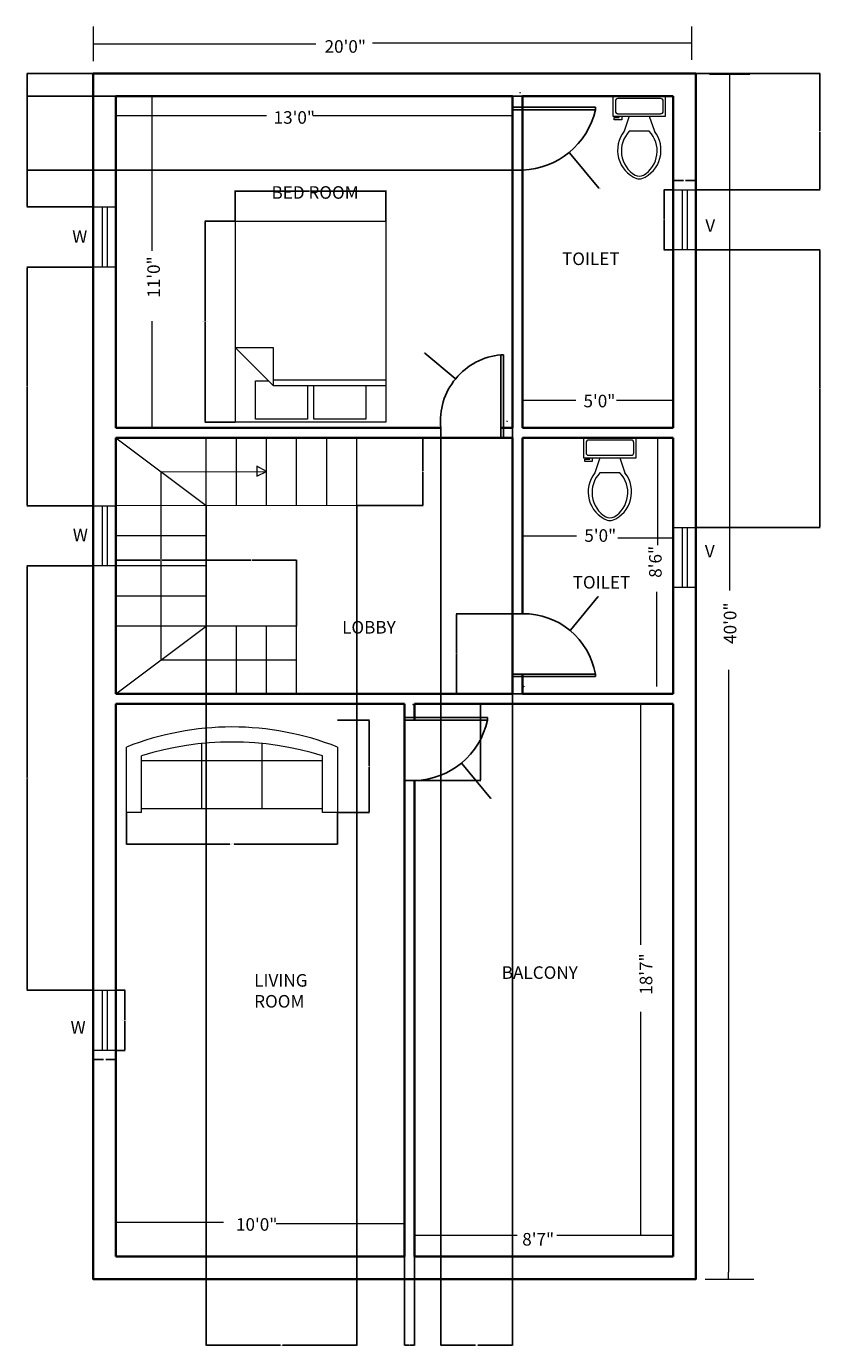
# Model space of a CAD drawing. Units: inches. Extents: x -58 to 719, y -488 to 73.
# Tile 3 of 3: x 403 to 719, y -488 to 37. Entities that reach past the tile are written whole.
import ezdxf

# ---------------------------------------------------------------- set-up
doc = ezdxf.new("R2010")
doc.units = ezdxf.units.IN
doc.header["$MEASUREMENT"] = 0
for name, color, linetype, lineweight in [('A-ANNO-DIMS', 2, 'Continuous', 13), ('A-ANNO-TEXT', 7, 'Continuous', 18), ('A-AREA-IDEN', 7, 'Continuous', 25), ('A-DOOR', 3, 'Continuous', 25), ('A-FLOR-FIXT', 9, 'Continuous', 18), ('A-FLOR-STRS', 7, 'Continuous', 18), ('A-FURN', 8, 'Continuous', 18), ('A-GLAZ', 4, 'Continuous', 18), ('A-WALL', 7, 'Continuous', 35)]:
    doc.layers.add(name, color=color, linetype=linetype, lineweight=lineweight)
doc.styles.get("Standard").update_dxf_attribs({"font": 'arial.ttf'})
doc.dimstyles.get("Standard").update_dxf_attribs({"dimtxt": 0.18, "dimasz": 0.18, "dimexe": 0.18, "dimexo": 0.0625, "dimgap": 0.09, "dimtad": 0, "dimtih": 1, "dimtoh": 1, "dimdec": 4, "dimzin": 0, "dimdsep": 46, "dimtxsty": 'Standard', "dimcen": 0.09, "dimadec": 0, "dimazin": 0, "dimtfac": 1, "dimtdec": 4, "dimtofl": 0, "dimtmove": 0, "dimatfit": 3, "dimfxl": 1, "dimtolj": 1, "dimtzin": 0, "dimarcsym": 0})

# ---------------------------------------------------------------- blocks, each defined once
blk = doc.blocks.new('Bed - Queen')
for p, q in [((0, -80.00003), (0, 0)), ((0, 0), (59.99999, 0)), ((59.99999, 0), (59.99999, -80.00003)), ((7.99999, -1.2), (28.79998, -1.2)), ((7.99999, -14.4), (7.99999, -1.2)), ((28.79998, -1.2), (28.79998, -14.4)), ((31.19999, -1.2), (51.99999, -1.2)), ((31.19999, -14.4), (31.19999, -1.2)), ((51.99999, -1.2), (51.99999, -16.4)), ((0, -14.4), (44.8, -14.4)), ((59.99999, -29.6), (44.8, -14.4)), ((44.8, -14.4), (44.8, -29.6)), ((44.8, -16.8), (0, -16.8)), ((51.99999, -16.4), (46.79936, -16.4)), ((44.8, -29.6), (59.99999, -29.6)), ((59.99999, -80.00003), (0, -80.00003))]:
    blk.add_line(p, q)
blk = doc.blocks.new('Toilet - top')
for p, q in [((9.5, -6), (9.5, -2)), ((-10, -8.5), (-8, -8.5)), ((-10, -9.5), (-10, -8.5)), ((-7, -9.5), (-10, -9.5)), ((-8, -8.5), (-8, -8)), ((-7, -8), (-7, -9.5)), ((-4, -8), (-6, -14)), ((4, -8), (6, -14)), ((4, -14), (-4, -14))]:
    blk.add_line(p, q)
blk.add_lwpolyline([(10.5, -8), (10.5, 0), (-10.5, 0), (-10.5, -8)], close=True)
for points in [[(-9.5, -2), (-9.5, -6)], [(8.5, -1), (-8.5, -1)], [(-8.5, -7), (8.5, -7)]]:
    blk.add_lwpolyline(points)
for centre, radius, start, end in [((-8.62, -1.88), 0.884, 81.8699, 188.1301), ((8.62, -1.88), 0.884, 351.8699, 98.1301), ((-8.62, -6.12), 0.884, 171.8699, 278.1301), ((8.62, -6.12), 0.884, 261.8699, 8.1301), ((3.52, -21.58), 12.17, 141.4691, 247.9714), ((4.2, -21.82), 11.33, 136.3677, 238.9468), ((-3.52, -21.58), 12.17, 292.0284, 38.5307), ((-4.2, -21.82), 11.33, 301.053, 43.6321), ((0, -27.88), 4, 245.7318, 294.2682), ((0, -29), 4, 254.8605, 285.1395)]:
    blk.add_arc(centre, radius, start, end)
blk = doc.blocks.new('Sofa - Roundback 7 ft.')
for p, q in [((-12.00002, -32.4421), (-12.00003, -6.5971)), ((11.99997, -32.4421), (11.99998, -6.5971)), ((-36.000027, -34), (-36.000027, -11.4696)), ((-35.999844, -13.3819), (35.9998, -13.3819)), ((35.99998, -34), (35.99998, -11.4696)), ((-36.000027, -32.4421), (35.99998, -32.4421))]:
    blk.add_line(p, q)
for points in [[(-36.000027, -34), (-42.000027, -34), (-42.000027, -8)], [(41.99998, -8), (41.99998, -34), (35.99998, -34)]]:
    blk.add_lwpolyline(points)
for centre, radius, start, end in [((0, -114.25), 114.25, 68.43141, 111.5686), ((-0.00001, -127.1968), 121.1968, 72.72033, 107.2797)]:
    blk.add_arc(centre, radius, start, end)
blk = doc.blocks.new('WIN-24IN')
for p, q in [((3.5, 24), (3.5, 0)), ((5.5, 24), (5.5, 0))]:
    blk.add_line(p, q)
blk.add_lwpolyline([(0, 24), (9, 24), (9, 0), (0, 0)], close=True)
blk = doc.blocks.new('VENT-24IN')
for p, q in [((3.5, 24), (3.5, 0)), ((5.5, 24), (5.5, 0))]:
    blk.add_line(p, q)
blk.add_lwpolyline([(0, 24), (9, 24), (9, 0), (0, 0)], close=True)
blk = doc.blocks.new('*D9')
at = {"layer": 'A-ANNO-DIMS', "color": 0, "lineweight": -2, "transparency": 16777216}
for p, q in [((438.81, -346.42), (442.52, -346.42)), ((442.34, -346.6), (442.34, -358.24)), ((442.34, -370.24), (442.34, -358.61)), ((438.81, -370.42), (442.52, -370.42))]:
    blk.add_line(p, q, dxfattribs=at)
at = {"layer": 'A-ANNO-DIMS', "color": 0, "transparency": 16777216}
for points in [[(442.31, -346.6), (442.37, -346.6), (442.34, -346.42)], [(442.31, -370.24), (442.37, -370.24), (442.34, -370.42)]]:
    blk.add_solid(points, dxfattribs=at)
at = {"layer": 'Defpoints', "color": 0, "transparency": 16777216}
for p in [(438.74, -346.42), (442.34, -346.42), (438.74, -370.42)]:
    blk.add_point(p, dxfattribs=at)
at = {"layer": 'A-ANNO-DIMS', "color": 0, "transparency": 16777216, "insert": (442.34, -358.42), "char_height": 0.18, "attachment_point": 5}
blk.add_mtext('\\A1;WINDOW 24 TYP.', dxfattribs=at)
blk = doc.blocks.new('*D10')
at = {"layer": 'A-ANNO-DIMS', "color": 0, "lineweight": -2, "transparency": 16777216}
for p, q in [((429.74, -370.49), (429.74, -374.2)), ((438.74, -370.49), (438.74, -374.2)), ((429.92, -374.02), (433.78, -374.02)), ((438.56, -374.02), (434.7, -374.02))]:
    blk.add_line(p, q, dxfattribs=at)
at = {"layer": 'A-ANNO-DIMS', "color": 0, "transparency": 16777216}
for points in [[(429.92, -373.99), (429.92, -374.05), (429.74, -374.02)], [(438.56, -373.99), (438.56, -374.05), (438.74, -374.02)]]:
    blk.add_solid(points, dxfattribs=at)
at = {"layer": 'Defpoints', "color": 0, "transparency": 16777216}
for p in [(429.74, -370.42), (438.74, -370.42), (438.74, -374.02)]:
    blk.add_point(p, dxfattribs=at)
at = {"layer": 'A-ANNO-DIMS', "color": 0, "transparency": 16777216, "insert": (434.24, -374.02), "char_height": 0.18, "attachment_point": 5}
blk.add_mtext('\\A1;9 TYP.', dxfattribs=at)
blk = doc.blocks.new('*D11')
at = {"layer": 'A-ANNO-DIMS', "color": 0, "lineweight": -2, "transparency": 16777216}
for p, q in [((660.68, -27.78), (656.96, -27.78)), ((657.14, -27.96), (657.14, -39.6)), ((657.14, -51.6), (657.14, -39.96)), ((660.68, -51.78), (656.96, -51.78))]:
    blk.add_line(p, q, dxfattribs=at)
at = {"layer": 'A-ANNO-DIMS', "color": 0, "transparency": 16777216}
for points in [[(657.11, -27.96), (657.17, -27.96), (657.14, -27.78)], [(657.11, -51.6), (657.17, -51.6), (657.14, -51.78)]]:
    blk.add_solid(points, dxfattribs=at)
at = {"layer": 'Defpoints', "color": 0, "transparency": 16777216}
for p in [(657.14, -27.78), (660.74, -27.78), (660.74, -51.78)]:
    blk.add_point(p, dxfattribs=at)
at = {"layer": 'A-ANNO-DIMS', "color": 0, "transparency": 16777216, "insert": (657.14, -39.78), "char_height": 0.18, "attachment_point": 5}
blk.add_mtext('\\A1;VENT 24 TYP.', dxfattribs=at)
blk = doc.blocks.new('*D12')
at = {"layer": 'A-ANNO-DIMS', "color": 0, "lineweight": -2, "transparency": 16777216}
for p, q in [((660.74, -27.72), (660.74, -24)), ((660.92, -24.18), (664.78, -24.18)), ((669.56, -24.18), (665.7, -24.18)), ((669.74, -27.72), (669.74, -24))]:
    blk.add_line(p, q, dxfattribs=at)
at = {"layer": 'A-ANNO-DIMS', "color": 0, "transparency": 16777216}
for points in [[(660.92, -24.15), (660.92, -24.21), (660.74, -24.18)], [(669.56, -24.15), (669.56, -24.21), (669.74, -24.18)]]:
    blk.add_solid(points, dxfattribs=at)
at = {"layer": 'Defpoints', "color": 0, "transparency": 16777216}
for p in [(669.74, -24.18), (660.74, -27.78), (669.74, -27.78)]:
    blk.add_point(p, dxfattribs=at)
at = {"layer": 'A-ANNO-DIMS', "color": 0, "transparency": 16777216, "insert": (665.24, -24.18), "char_height": 0.18, "attachment_point": 5}
blk.add_mtext('\\A1;9 TYP.', dxfattribs=at)
blk = doc.blocks.new('*D15')
at = {"layer": 'A-ANNO-DIMS', "color": 0, "lineweight": -2, "transparency": 16777216}
for p, q in [((486.28, -40.31), (474.16, -40.31)), ((474.34, -40.49), (474.34, -80.12)), ((474.34, -120.13), (474.34, -80.5)), ((486.28, -120.31), (474.16, -120.31))]:
    blk.add_line(p, q, dxfattribs=at)
at = {"layer": 'A-ANNO-DIMS', "color": 0, "transparency": 16777216}
for points in [[(474.31, -40.49), (474.37, -40.49), (474.34, -40.31)], [(474.31, -120.13), (474.37, -120.13), (474.34, -120.31)]]:
    blk.add_solid(points, dxfattribs=at)
at = {"layer": 'Defpoints', "color": 0, "transparency": 16777216}
for p in [(486.34, -40.31), (474.34, -120.31), (486.34, -120.31)]:
    blk.add_point(p, dxfattribs=at)
at = {"layer": 'A-ANNO-DIMS', "color": 0, "transparency": 16777216, "insert": (474.34, -80.31), "char_height": 0.18, "attachment_point": 5}
blk.add_mtext('\\A1;QUEEN BED 80 TYP.', dxfattribs=at)
blk = doc.blocks.new('*D16')
at = {"layer": 'A-ANNO-DIMS', "color": 0, "lineweight": -2, "transparency": 16777216}
for p, q in [((486.34, -40.25), (486.34, -28.13)), ((486.52, -28.31), (515.82, -28.31)), ((546.16, -28.31), (516.87, -28.31)), ((546.34, -40.25), (546.34, -28.13))]:
    blk.add_line(p, q, dxfattribs=at)
at = {"layer": 'A-ANNO-DIMS', "color": 0, "transparency": 16777216}
for points in [[(486.52, -28.28), (486.52, -28.34), (486.34, -28.31)], [(546.16, -28.28), (546.16, -28.34), (546.34, -28.31)]]:
    blk.add_solid(points, dxfattribs=at)
at = {"layer": 'Defpoints', "color": 0, "transparency": 16777216}
for p in [(486.34, -28.31), (486.34, -40.31), (546.34, -40.31)]:
    blk.add_point(p, dxfattribs=at)
at = {"layer": 'A-ANNO-DIMS', "color": 0, "transparency": 16777216, "insert": (516.34, -28.31), "char_height": 0.18, "attachment_point": 5}
blk.add_mtext('\\A1;60 TYP.', dxfattribs=at)
blk = doc.blocks.new('*D17')
at = {"layer": 'A-ANNO-DIMS', "color": 0, "lineweight": -2, "transparency": 16777216}
for p, q in [((443.01, -275.74), (443.01, -288.46)), ((527.01, -275.74), (527.01, -288.46)), ((443.19, -288.28), (484.1, -288.28)), ((526.83, -288.28), (485.91, -288.28))]:
    blk.add_line(p, q, dxfattribs=at)
at = {"layer": 'A-ANNO-DIMS', "color": 0, "transparency": 16777216}
for points in [[(443.19, -288.25), (443.19, -288.31), (443.01, -288.28)], [(526.83, -288.25), (526.83, -288.31), (527.01, -288.28)]]:
    blk.add_solid(points, dxfattribs=at)
at = {"layer": 'Defpoints', "color": 0, "transparency": 16777216}
for p in [(443.01, -275.68), (527.01, -275.68), (527.01, -288.28)]:
    blk.add_point(p, dxfattribs=at)
at = {"layer": 'A-ANNO-DIMS', "color": 0, "transparency": 16777216, "insert": (485.01, -288.28), "char_height": 0.18, "attachment_point": 5}
blk.add_mtext('\\A1;SOFA 84 TYP.', dxfattribs=at)
blk = doc.blocks.new('*D18')
at = {"layer": 'A-ANNO-DIMS', "color": 0, "lineweight": -2, "transparency": 16777216}
for p, q in [((527.07, -239.01), (539.79, -239.01)), ((539.61, -239.19), (539.61, -257.16)), ((539.61, -275.5), (539.61, -257.53)), ((527.07, -275.68), (539.79, -275.68))]:
    blk.add_line(p, q, dxfattribs=at)
at = {"layer": 'A-ANNO-DIMS', "color": 0, "transparency": 16777216}
for points in [[(539.58, -239.19), (539.64, -239.19), (539.61, -239.01)], [(539.58, -275.5), (539.64, -275.5), (539.61, -275.68)]]:
    blk.add_solid(points, dxfattribs=at)
at = {"layer": 'Defpoints', "color": 0, "transparency": 16777216}
for p in [(527.01, -239.01), (539.61, -239.01), (527.01, -275.68)]:
    blk.add_point(p, dxfattribs=at)
at = {"layer": 'A-ANNO-DIMS', "color": 0, "transparency": 16777216, "insert": (539.61, -257.34), "char_height": 0.18, "attachment_point": 5}
blk.add_mtext('\\A1;37 TYP.', dxfattribs=at)
blk = doc.blocks.new('*D33')
at = {"layer": 'A-ANNO-DIMS', "color": 0, "lineweight": -2, "transparency": 16777216}
for p, q in [((429.68, 18.48), (403.31, 18.48)), ((403.49, 18.3), (403.49, -7.91)), ((403.49, -34.48), (403.49, -8.27)), ((429.68, -34.66), (403.31, -34.66))]:
    blk.add_line(p, q, dxfattribs=at)
at = {"layer": 'A-ANNO-DIMS', "color": 0, "transparency": 16777216}
for points in [[(403.46, 18.3), (403.52, 18.3), (403.49, 18.48)], [(403.46, -34.48), (403.52, -34.48), (403.49, -34.66)]]:
    blk.add_solid(points, dxfattribs=at)
at = {"layer": 'Defpoints', "color": 0, "transparency": 16777216}
for p in [(429.74, 18.48), (403.49, -34.66), (429.74, -34.66)]:
    blk.add_point(p, dxfattribs=at)
at = {"layer": 'A-ANNO-DIMS', "color": 0, "transparency": 16777216, "insert": (403.49, -8.09), "char_height": 0.18, "attachment_point": 5}
blk.add_mtext('\\A1;53.14', dxfattribs=at)
blk = doc.blocks.new('*D34')
at = {"layer": 'A-ANNO-DIMS', "color": 0, "lineweight": -2, "transparency": 16777216}
for p, q in [((429.68, -58.66), (403.31, -58.66)), ((403.49, -58.84), (403.49, -105.94)), ((403.49, -153.4), (403.49, -106.3)), ((429.68, -153.58), (403.31, -153.58))]:
    blk.add_line(p, q, dxfattribs=at)
at = {"layer": 'A-ANNO-DIMS', "color": 0, "transparency": 16777216}
for points in [[(403.46, -58.84), (403.52, -58.84), (403.49, -58.66)], [(403.46, -153.4), (403.52, -153.4), (403.49, -153.58)]]:
    blk.add_solid(points, dxfattribs=at)
at = {"layer": 'Defpoints', "color": 0, "transparency": 16777216}
for p in [(429.74, -58.66), (403.49, -153.58), (429.74, -153.58)]:
    blk.add_point(p, dxfattribs=at)
at = {"layer": 'A-ANNO-DIMS', "color": 0, "transparency": 16777216, "insert": (403.49, -106.12), "char_height": 0.18, "attachment_point": 5}
blk.add_mtext('\\A1;94.93', dxfattribs=at)
blk = doc.blocks.new('*D35')
at = {"layer": 'A-ANNO-DIMS', "color": 0, "lineweight": -2, "transparency": 16777216}
for p, q in [((429.68, -177.58), (403.31, -177.58)), ((403.49, -177.76), (403.49, -261.82)), ((403.49, -346.24), (403.49, -262.19)), ((429.68, -346.42), (403.31, -346.42))]:
    blk.add_line(p, q, dxfattribs=at)
at = {"layer": 'A-ANNO-DIMS', "color": 0, "transparency": 16777216}
for points in [[(403.46, -177.76), (403.52, -177.76), (403.49, -177.58)], [(403.46, -346.24), (403.52, -346.24), (403.49, -346.42)]]:
    blk.add_solid(points, dxfattribs=at)
at = {"layer": 'Defpoints', "color": 0, "transparency": 16777216}
for p in [(429.74, -177.58), (403.49, -346.42), (429.74, -346.42)]:
    blk.add_point(p, dxfattribs=at)
at = {"layer": 'A-ANNO-DIMS', "color": 0, "transparency": 16777216, "insert": (403.49, -262), "char_height": 0.18, "attachment_point": 5}
blk.add_mtext('\\A1;168.84', dxfattribs=at)
blk = doc.blocks.new('*D36')
at = {"layer": 'A-ANNO-DIMS', "color": 0, "lineweight": -2, "transparency": 16777216}
for p, q in [((669.81, 18.48), (719.26, 18.48)), ((719.08, 18.3), (719.08, -4.47)), ((719.08, -27.6), (719.08, -4.83)), ((669.81, -27.78), (719.26, -27.78))]:
    blk.add_line(p, q, dxfattribs=at)
at = {"layer": 'A-ANNO-DIMS', "color": 0, "transparency": 16777216}
for points in [[(719.05, 18.3), (719.11, 18.3), (719.08, 18.48)], [(719.05, -27.6), (719.11, -27.6), (719.08, -27.78)]]:
    blk.add_solid(points, dxfattribs=at)
at = {"layer": 'Defpoints', "color": 0, "transparency": 16777216}
for p in [(669.74, 18.48), (669.74, -27.78), (719.08, -27.78)]:
    blk.add_point(p, dxfattribs=at)
at = {"layer": 'A-ANNO-DIMS', "color": 0, "transparency": 16777216, "insert": (719.08, -4.65), "char_height": 0.18, "attachment_point": 5}
blk.add_mtext('\\A1;46.26', dxfattribs=at)
blk = doc.blocks.new('*D37')
at = {"layer": 'A-ANNO-DIMS', "color": 0, "lineweight": -2, "transparency": 16777216}
for p, q in [((669.81, -51.78), (719.26, -51.78)), ((719.08, -51.96), (719.08, -106.81)), ((719.08, -162.03), (719.08, -107.18)), ((669.81, -162.21), (719.26, -162.21))]:
    blk.add_line(p, q, dxfattribs=at)
at = {"layer": 'A-ANNO-DIMS', "color": 0, "transparency": 16777216}
for points in [[(719.05, -51.96), (719.11, -51.96), (719.08, -51.78)], [(719.05, -162.03), (719.11, -162.03), (719.08, -162.21)]]:
    blk.add_solid(points, dxfattribs=at)
at = {"layer": 'Defpoints', "color": 0, "transparency": 16777216}
for p in [(669.74, -51.78), (669.74, -162.21), (719.08, -162.21)]:
    blk.add_point(p, dxfattribs=at)
at = {"layer": 'A-ANNO-DIMS', "color": 0, "transparency": 16777216, "insert": (719.08, -106.99), "char_height": 0.18, "attachment_point": 5}
blk.add_mtext('\\A1;110.43', dxfattribs=at)
blk = doc.blocks.new('*D45')
at = {"layer": 'A-ANNO-DIMS', "color": 0, "lineweight": -2, "transparency": 16777216}
for p, q in [((438.76, -201.52), (438.74, -175.15)), ((438.92, -175.33), (456.27, -175.32)), ((474.55, -175.31), (457.2, -175.32)), ((474.74, -201.5), (474.73, -175.13))]:
    blk.add_line(p, q, dxfattribs=at)
at = {"layer": 'A-ANNO-DIMS', "color": 0, "transparency": 16777216}
for points in [[(438.92, -175.3), (438.92, -175.36), (438.74, -175.33)], [(474.55, -175.28), (474.55, -175.34), (474.73, -175.31)]]:
    blk.add_solid(points, dxfattribs=at)
at = {"layer": 'Defpoints', "color": 0, "transparency": 16777216}
for p in [(474.73, -175.31), (438.76, -201.58), (474.74, -201.56)]:
    blk.add_point(p, dxfattribs=at)
at = {"layer": 'A-ANNO-DIMS', "color": 0, "transparency": 16777216, "insert": (456.73, -175.32), "char_height": 0.18, "attachment_point": 5}
blk.add_mtext('\\A1;35.985', dxfattribs=at)
blk = doc.blocks.new('*D46')
at = {"layer": 'A-ANNO-DIMS', "color": 0, "lineweight": -2, "transparency": 16777216}
for p, q in [((534.81, -126.52), (561.17, -126.54)), ((560.99, -126.72), (560.99, -139.86)), ((560.98, -153.36), (560.99, -140.22)), ((534.79, -153.52), (561.16, -153.54))]:
    blk.add_line(p, q, dxfattribs=at)
at = {"layer": 'A-ANNO-DIMS', "color": 0, "transparency": 16777216}
for points in [[(560.96, -126.72), (561.02, -126.72), (560.99, -126.54)], [(560.95, -153.36), (561.01, -153.36), (560.98, -153.54)]]:
    blk.add_solid(points, dxfattribs=at)
at = {"layer": 'Defpoints', "color": 0, "transparency": 16777216}
for p in [(534.74, -126.52), (534.73, -153.52), (560.98, -153.54)]:
    blk.add_point(p, dxfattribs=at)
at = {"layer": 'A-ANNO-DIMS', "color": 0, "transparency": 16777216, "insert": (560.99, -140.04), "char_height": 0.18, "attachment_point": 5}
blk.add_mtext('\\A1;27', dxfattribs=at)
blk = doc.blocks.new('*D47')
at = {"layer": 'A-ANNO-DIMS', "color": 0, "lineweight": -2, "transparency": 16777216}
for p, q in [((474.74, -153.62), (474.74, -487.95)), ((534.73, -153.59), (534.73, -487.95)), ((474.92, -487.77), (504.34, -487.77)), ((534.55, -487.77), (505.13, -487.77))]:
    blk.add_line(p, q, dxfattribs=at)
at = {"layer": 'A-ANNO-DIMS', "color": 0, "transparency": 16777216}
for points in [[(474.92, -487.74), (474.92, -487.8), (474.74, -487.77)], [(534.55, -487.74), (534.55, -487.8), (534.73, -487.77)]]:
    blk.add_solid(points, dxfattribs=at)
at = {"layer": 'Defpoints', "color": 0, "transparency": 16777216}
for p in [(474.74, -153.56), (534.73, -153.52), (534.73, -487.77)]:
    blk.add_point(p, dxfattribs=at)
at = {"layer": 'A-ANNO-DIMS', "color": 0, "transparency": 16777216, "insert": (504.74, -487.77), "char_height": 0.18, "attachment_point": 5}
blk.add_mtext('\\A1;59.98', dxfattribs=at)
blk = doc.blocks.new('*D48')
at = {"layer": 'A-ANNO-DIMS', "color": 0, "lineweight": -2, "transparency": 16777216}
for p, q in [((474.74, -201.5), (474.73, -175.13)), ((474.91, -175.31), (492.51, -175.3)), ((510.55, -175.29), (492.95, -175.3)), ((510.74, -201.48), (510.73, -175.11))]:
    blk.add_line(p, q, dxfattribs=at)
at = {"layer": 'A-ANNO-DIMS', "color": 0, "transparency": 16777216}
for points in [[(474.91, -175.28), (474.91, -175.34), (474.73, -175.31)], [(510.55, -175.26), (510.55, -175.32), (510.73, -175.29)]]:
    blk.add_solid(points, dxfattribs=at)
at = {"layer": 'Defpoints', "color": 0, "transparency": 16777216}
for p in [(510.73, -175.29), (474.74, -201.56), (510.74, -201.54)]:
    blk.add_point(p, dxfattribs=at)
at = {"layer": 'A-ANNO-DIMS', "color": 0, "transparency": 16777216, "insert": (492.73, -175.3), "char_height": 0.18, "attachment_point": 5}
blk.add_mtext('\\A1;36', dxfattribs=at)
blk = doc.blocks.new('*D53')
at = {"layer": 'A-ANNO-DIMS', "color": 0, "lineweight": -2, "transparency": 16777216}
for p, q in [((568.13, -122.59), (568.13, -487.95)), ((596.74, -122.59), (596.74, -487.95)), ((568.31, -487.77), (581.97, -487.77)), ((596.56, -487.77), (582.9, -487.77))]:
    blk.add_line(p, q, dxfattribs=at)
at = {"layer": 'A-ANNO-DIMS', "color": 0, "transparency": 16777216}
for points in [[(568.31, -487.74), (568.31, -487.8), (568.13, -487.77)], [(596.56, -487.74), (596.56, -487.8), (596.74, -487.77)]]:
    blk.add_solid(points, dxfattribs=at)
at = {"layer": 'Defpoints', "color": 0, "transparency": 16777216}
for p in [(568.13, -122.52), (596.74, -122.52), (596.74, -487.77)]:
    blk.add_point(p, dxfattribs=at)
at = {"layer": 'A-ANNO-DIMS', "color": 0, "transparency": 16777216, "insert": (582.44, -487.77), "char_height": 0.18, "attachment_point": 5}
blk.add_mtext('\\A1;28.616', dxfattribs=at)
blk = doc.blocks.new('*D54')
at = {"layer": 'A-ANNO-DIMS', "color": 0, "lineweight": -2, "transparency": 16777216}
for p, q in [((600.68, 9.48), (403.31, 9.48)), ((403.49, 9.3), (403.49, -5.06)), ((403.49, -19.78), (403.49, -5.43)), ((600.68, -19.96), (403.31, -19.96))]:
    blk.add_line(p, q, dxfattribs=at)
at = {"layer": 'A-ANNO-DIMS', "color": 0, "transparency": 16777216}
for points in [[(403.46, 9.3), (403.52, 9.3), (403.49, 9.48)], [(403.46, -19.78), (403.52, -19.78), (403.49, -19.96)]]:
    blk.add_solid(points, dxfattribs=at)
at = {"layer": 'Defpoints', "color": 0, "transparency": 16777216}
for p in [(600.74, 9.48), (403.49, -19.96), (600.74, -19.96)]:
    blk.add_point(p, dxfattribs=at)
at = {"layer": 'A-ANNO-DIMS', "color": 0, "transparency": 16777216, "insert": (403.49, -5.24), "char_height": 0.18, "attachment_point": 5}
blk.add_mtext('\\A1;29.44', dxfattribs=at)
blk = doc.blocks.new('*D55')
at = {"layer": 'A-ANNO-DIMS', "color": 0, "lineweight": -2, "transparency": 16777216}
for p, q in [((600.68, -196.62), (574.31, -196.62)), ((574.49, -196.8), (574.49, -212.39)), ((574.49, -228.34), (574.49, -212.75)), ((600.68, -228.52), (574.31, -228.52))]:
    blk.add_line(p, q, dxfattribs=at)
at = {"layer": 'A-ANNO-DIMS', "color": 0, "transparency": 16777216}
for points in [[(574.46, -196.8), (574.52, -196.8), (574.49, -196.62)], [(574.46, -228.34), (574.52, -228.34), (574.49, -228.52)]]:
    blk.add_solid(points, dxfattribs=at)
at = {"layer": 'Defpoints', "color": 0, "transparency": 16777216}
for p in [(574.49, -196.62), (600.74, -196.62), (600.74, -228.52)]:
    blk.add_point(p, dxfattribs=at)
at = {"layer": 'A-ANNO-DIMS', "color": 0, "transparency": 16777216, "insert": (574.49, -212.57), "char_height": 0.18, "attachment_point": 5}
blk.add_mtext('\\A1;31.9', dxfattribs=at)
blk = doc.blocks.new('*D56')
at = {"layer": 'A-ANNO-DIMS', "color": 0, "lineweight": -2, "transparency": 16777216}
for p, q in [((557.81, -232.52), (584.17, -232.52)), ((583.99, -232.7), (583.99, -247.56)), ((583.99, -262.77), (583.99, -247.92)), ((557.81, -262.95), (584.17, -262.95))]:
    blk.add_line(p, q, dxfattribs=at)
at = {"layer": 'A-ANNO-DIMS', "color": 0, "transparency": 16777216}
for points in [[(583.96, -232.7), (584.02, -232.7), (583.99, -232.52)], [(583.96, -262.77), (584.02, -262.77), (583.99, -262.95)]]:
    blk.add_solid(points, dxfattribs=at)
at = {"layer": 'Defpoints', "color": 0, "transparency": 16777216}
for p in [(557.74, -232.52), (557.74, -262.95), (583.99, -262.95)]:
    blk.add_point(p, dxfattribs=at)
at = {"layer": 'A-ANNO-DIMS', "color": 0, "transparency": 16777216, "insert": (583.99, -247.74), "char_height": 0.18, "attachment_point": 5}
blk.add_mtext('\\A1;30.43', dxfattribs=at)
blk = doc.blocks.new('*D58')
at = {"layer": 'A-ANNO-DIMS', "color": 0, "lineweight": -2, "transparency": 16777216}
for p, q in [((553.74, -452.59), (553.74, -487.95)), ((557.74, -452.59), (557.74, -487.95)), ((553.92, -487.77), (555.59, -487.77)), ((557.56, -487.77), (555.9, -487.77))]:
    blk.add_line(p, q, dxfattribs=at)
at = {"layer": 'A-ANNO-DIMS', "color": 0, "transparency": 16777216}
for points in [[(553.92, -487.74), (553.92, -487.8), (553.74, -487.77)], [(557.56, -487.74), (557.56, -487.8), (557.74, -487.77)]]:
    blk.add_solid(points, dxfattribs=at)
at = {"layer": 'Defpoints', "color": 0, "transparency": 16777216}
for p in [(553.74, -452.52), (557.74, -452.52), (557.74, -487.77)]:
    blk.add_point(p, dxfattribs=at)
at = {"layer": 'A-ANNO-DIMS', "color": 0, "transparency": 16777216, "insert": (555.74, -487.77), "char_height": 0.18, "attachment_point": 5}
blk.add_mtext('\\A1;4', dxfattribs=at)
blk = doc.blocks.new('*D64')
at = {"layer": 'A-ANNO-DIMS', "color": 0, "lineweight": -2, "transparency": 16777216}
for p, q in [((599.63, 10.8), (599.81, 10.8)), ((599.72, 10.71), (599.72, 10.89)), ((631.11, -27.14), (619.45, -13.05)), ((631.29, -27.14), (631.11, -27.14))]:
    blk.add_line(p, q, dxfattribs=at)
at = {"layer": 'A-ANNO-DIMS', "color": 0, "transparency": 16777216}
blk.add_solid([(619.48, -13.03), (619.43, -13.07), (619.34, -12.91)], dxfattribs=at)
at = {"layer": 'Defpoints', "color": 0, "transparency": 16777216}
for p in [(599.72, 10.8), (619.34, -12.91)]:
    blk.add_point(p, dxfattribs=at)
at = {"layer": 'A-ANNO-DIMS', "color": 0, "transparency": 16777216, "insert": (631.84, -27.14), "char_height": 0.18, "attachment_point": 5}
blk.add_mtext('\\A1;R30.775', dxfattribs=at)
blk = doc.blocks.new('*D65')
at = {"layer": 'A-ANNO-DIMS', "color": 0, "lineweight": -2, "transparency": 16777216}
for p, q in [((557.1, -232.76), (557.28, -232.76)), ((557.19, -232.85), (557.19, -232.67)), ((587.99, -269.98), (576.56, -256.16)), ((588.17, -269.98), (587.99, -269.98))]:
    blk.add_line(p, q, dxfattribs=at)
at = {"layer": 'A-ANNO-DIMS', "color": 0, "transparency": 16777216}
blk.add_solid([(576.58, -256.14), (576.53, -256.18), (576.44, -256.02)], dxfattribs=at)
at = {"layer": 'Defpoints', "color": 0, "transparency": 16777216}
for p in [(557.19, -232.76), (576.44, -256.02)]:
    blk.add_point(p, dxfattribs=at)
at = {"layer": 'A-ANNO-DIMS', "color": 0, "transparency": 16777216, "insert": (588.65, -269.98), "char_height": 0.18, "attachment_point": 5}
blk.add_mtext('\\A1;R30.19', dxfattribs=at)
blk = doc.blocks.new('*D66')
at = {"layer": 'A-ANNO-DIMS', "color": 0, "lineweight": -2, "transparency": 16777216}
for p, q in [((630.75, -189.89), (619.79, -203.13)), ((630.93, -189.89), (630.75, -189.89)), ((601.13, -225.56), (601.31, -225.56)), ((601.22, -225.65), (601.22, -225.47))]:
    blk.add_line(p, q, dxfattribs=at)
at = {"layer": 'A-ANNO-DIMS', "color": 0, "transparency": 16777216}
blk.add_solid([(619.77, -203.11), (619.82, -203.14), (619.68, -203.26)], dxfattribs=at)
at = {"layer": 'Defpoints', "color": 0, "transparency": 16777216}
for p in [(619.68, -203.26), (601.22, -225.56)]:
    blk.add_point(p, dxfattribs=at)
at = {"layer": 'A-ANNO-DIMS', "color": 0, "transparency": 16777216, "insert": (631.48, -189.89), "char_height": 0.18, "attachment_point": 5}
blk.add_mtext('\\A1;R28.943', dxfattribs=at)
blk = doc.blocks.new('*D67')
at = {"layer": 'A-ANNO-DIMS', "color": 0, "lineweight": -2, "transparency": 16777216}
for p, q in [((561.65, -92.88), (561.83, -92.88)), ((561.83, -92.88), (573.96, -102.92)), ((594.46, -119.96), (594.64, -119.96)), ((594.55, -120.05), (594.55, -119.87))]:
    blk.add_line(p, q, dxfattribs=at)
at = {"layer": 'A-ANNO-DIMS', "color": 0, "transparency": 16777216}
blk.add_solid([(573.98, -102.9), (573.94, -102.94), (574.1, -103.03)], dxfattribs=at)
at = {"layer": 'Defpoints', "color": 0, "transparency": 16777216}
for p in [(574.1, -103.03), (594.55, -119.96)]:
    blk.add_point(p, dxfattribs=at)
at = {"layer": 'A-ANNO-DIMS', "color": 0, "transparency": 16777216, "insert": (561.17, -92.88), "char_height": 0.18, "attachment_point": 5}
blk.add_mtext('\\A1;R26.55', dxfattribs=at)

msp = doc.modelspace()

# ---------------------------------------------------------------- linework, layer by layer
at = {"layer": 'A-ANNO-DIMS'}
for p, q in [((429.8656, 23.3945), (429.8656, 37.2256)), ((667.9839, 37.2256), (667.9839, 23.9369)), ((429.8656, 30.31), (518.3794, 30.31)), ((540.9151, 30.7168), (667.9839, 30.7168)), ((675.1295, 18.1739), (691.2652, 18.1739)), ((683.1974, 18.1739), (683.1974, -187.3966)), ((453.1227, 9.477), (453.1227, -52.1073)), ((438.7431, 1.7137), (498.7389, 1.7137)), ((517.1677, 1.7137), (596.7431, 1.7137)), ((453.1227, -80.1252), (453.1227, -117.3293)), ((600.7431, -111.523), (621.9735, -111.523)), ((638.2182, -111.523), (660.7431, -111.523)), ((453.1227, -117.3293), (453.1227, -122.523)), ((654.426, -126.523), (654.426, -169.2515)), ((622.1908, -165.7576), (600.7431, -165.7576)), ((638.7421, -166.4191), (660.7431, -166.4191)), ((654.134, -187.9183), (654.134, -225.5434)), ((682.6971, -218.9281), (682.6971, -458.7791)), ((647.7609, -232.523), (647.7609, -328.4036)), ((647.7609, -355.0655), (647.7609, -443.9812)), ((438.7431, -438.7631), (481.5653, -438.7631)), ((502.6605, -439.3176), (553.7431, -439.3176)), ((557.7431, -443.9812), (598.62, -443.9812)), ((614.3405, -443.9812), (660.7431, -443.9812)), ((673.4797, -461.523), (682.6971, -461.523)), ((682.6971, -461.523), (682.6971, -458.7791)), ((682.6971, -461.523), (692.8287, -461.523))]:
    msp.add_line(p, q, dxfattribs=at)
at = {"layer": 'A-DOOR'}
for p, q in [((596.7431, 5.0367), (629.7431, 5.0367)), ((629.7431, 4.0367), (596.7431, 4.0367)), ((629.7431, 5.0367), (629.7431, 4.0367)), ((600.7431, -19.9633), (596.7431, -19.9633)), ((593.1272, -93.523), (592.1272, -93.523)), ((592.1272, -93.523), (592.1272, -126.523)), ((593.1272, -126.523), (593.1272, -93.523)), ((568.1272, -122.523), (568.1272, -126.523)), ((600.7431, -196.6222), (596.7431, -196.6222)), ((629.7431, -220.6222), (596.7431, -220.6222)), ((596.7431, -221.6222), (629.7431, -221.6222)), ((629.7431, -221.6222), (629.7431, -220.6222)), ((553.7431, -237.9512), (586.7431, -237.9512)), ((586.7431, -238.9512), (553.7431, -238.9512)), ((586.7431, -237.9512), (586.7431, -238.9512)), ((557.7431, -262.9512), (553.7431, -262.9512))]:
    msp.add_line(p, q, dxfattribs=at)
for centre, radius, start, end in [((599.7189, 10.7951), 30.7755, 271.90715, 347.314227), ((594.5526, -119.9612), 26.5493, 95.241577, 185.537046), ((601.2247, -225.5612), 28.943, 9.825331, 90.953292), ((557.1924, -232.7648), 30.1914, 271.045284, 348.176093)]:
    msp.add_arc(centre, radius, start, end, dxfattribs=at)
at = {"layer": 'A-FLOR-STRS'}
for p, q in [((438.7431, -126.523), (474.7431, -153.5612)), ((474.7431, -228.523), (474.7431, -126.523)), ((486.7431, -153.5536), (486.7431, -126.523)), ((498.7431, -153.5459), (498.7431, -126.523)), ((510.7431, -153.5383), (510.7431, -126.523)), ((522.7431, -153.5306), (522.7431, -126.523)), ((534.7278, -153.523), (534.7431, -126.523)), ((456.7431, -140.0421), (498.7431, -140.0344)), ((456.7431, -215.0421), (456.7431, -140.0421)), ((494.942, -137.8929), (494.942, -141.8819)), ((498.7431, -140.0344), (494.942, -137.8929)), ((494.942, -141.8819), (498.7431, -140.0344)), ((534.7278, -153.523), (438.7278, -153.5842)), ((474.7431, -165.5612), (438.7355, -165.5842)), ((474.7431, -177.5612), (438.7431, -177.5842)), ((474.7431, -189.5612), (438.7508, -189.5842)), ((438.7431, -228.523), (474.7431, -201.5612)), ((510.7431, -201.5383), (438.7584, -201.5842)), ((486.7431, -228.523), (486.7431, -201.5536)), ((498.7431, -228.523), (498.7431, -201.5459)), ((510.7431, -228.523), (510.7431, -201.5383)), ((510.7431, -215.0306), (456.7431, -215.0421))]:
    msp.add_line(p, q, dxfattribs=at)
at = {"layer": 'A-WALL'}
for p, q in [((438.7431, 9.477), (596.7431, 9.477)), ((438.7431, -122.523), (438.7431, 9.477)), ((596.7431, 9.477), (596.7431, -122.523)), ((600.7431, 9.477), (600.7431, -122.523)), ((600.7431, 9.477), (660.7431, 9.477)), ((660.7431, 9.477), (660.7431, -122.523)), ((438.7431, -122.523), (568.1272, -122.523)), ((592.1272, -122.523), (596.7431, -122.523)), ((600.7431, -122.523), (660.7431, -122.523)), ((438.7431, -126.523), (596.7431, -126.523)), ((438.7431, -228.523), (438.7431, -126.523)), ((596.7431, -126.523), (596.7431, -228.523)), ((600.7431, -126.523), (660.7431, -126.523)), ((600.7431, -126.523), (600.7431, -196.6222)), ((660.7431, -126.523), (660.7431, -228.523)), ((600.7431, -220.6222), (600.7431, -228.523)), ((438.7431, -228.523), (596.7431, -228.523)), ((600.7431, -228.523), (660.7431, -228.523)), ((438.7431, -452.523), (438.7431, -232.523)), ((438.7431, -232.523), (553.7431, -232.523)), ((553.7431, -232.523), (553.7431, -452.523)), ((557.7431, -232.523), (557.7431, -238.9512)), ((557.7431, -232.523), (660.7431, -232.523)), ((660.7431, -232.523), (660.7431, -452.523)), ((557.7431, -262.9512), (557.7431, -452.523)), ((553.7431, -452.523), (438.7431, -452.523)), ((660.7431, -452.523), (557.7431, -452.523))]:
    msp.add_line(p, q, dxfattribs=at)
msp.add_lwpolyline([(429.7431, 18.477), (669.7431, 18.477), (669.7431, -461.523), (429.7431, -461.523)], close=True, dxfattribs=at)

# ---------------------------------------------------------------- block references
at = {"layer": 'A-FLOR-FIXT'}
for p in [(647.2274, 9.477), (635.5266, -126.523)]:
    msp.add_blockref('Toilet - top', p, dxfattribs=at)
at = {"layer": 'A-FURN', "rotation": 180}
msp.add_blockref('Bed - Queen', (546.3439, -120.3101), dxfattribs=at)
at = {"layer": 'A-FURN'}
msp.add_blockref('Sofa - Roundback 7 ft.', (485.0061, -241.6778), dxfattribs=at)
at = {"layer": 'A-GLAZ'}
for name, p in [('VENT-24IN', (660.7427, -51.7791)), ('WIN-24IN', (429.7427, -58.6591)), ('WIN-24IN', (429.7427, -177.5841)), ('VENT-24IN', (660.7427, -186.2085)), ('WIN-24IN', (429.7427, -370.4228))]:
    msp.add_blockref(name, p, dxfattribs=at)

# ---------------------------------------------------------------- texts
at = {"layer": 'A-ANNO-DIMS', "char_height": 5, "attachment_point": 1}
for s, width, insert in [('20\'0"', 39.293008, (521.8841, 31.7285)), ('13\'0"', 18.031716, (501.5905, 3.4694)), ('5\'0"', 18.979899, (625.0034, -109.4175)), ('5\'0"', 19.842618, (625.3383, -162.9649)), ('10\'0"', 29.332567, (486.604, -437.2203)), ('8\'7"', 28.901213, (600.6037, -443.117))]:
    msp.add_mtext_dynamic_manual_height_columns(s, width=width, gutter_width=25, heights=[0], dxfattribs=dict(at, insert=insert))
at = {"layer": 'A-ANNO-DIMS', "char_height": 5, "attachment_point": 1, "rotation": 90}
for s, width, insert in [('11\'0"', 12.940832, (451.3061, -70.7987)), ('8\'6"', 13.803561, (651.137, -182.2878)), ('40\'0"', 39.717859, (680.8995, -208.6003)), ('18\'7"', 16.391725, (647.4232, -348.284))]:
    msp.add_mtext_dynamic_manual_height_columns(s, width=width, gutter_width=25, heights=[0], dxfattribs=dict(at, insert=insert))
at = {"layer": 'A-ANNO-TEXT', "char_height": 5, "attachment_point": 1}
for s, width, insert in [('V', 8.195867, (673.5282, -39.5472)), ('W', 7.804777, (421.383, -43.9)), ('W', 6.456169, (421.634, -162.7367)), ('V', 6.20876, (673.3428, -169.2082)), ('W', 16.342594, (420.7336, -358.75))]:
    msp.add_mtext_dynamic_manual_height_columns(s, width=width, gutter_width=25, heights=[0], dxfattribs=dict(at, insert=insert))
at = {"layer": 'A-AREA-IDEN', "char_height": 5, "attachment_point": 1}
for s, width, insert in [('BED ROOM', 45.292938, (500.739, -26.3925)), ('TOILET', 28.901203, (616.4527, -52.7868)), ('TOILET', 27.175767, (620.6925, -181.5854)), ('LOBBY', 48.312467, (528.8737, -199.4964)), ('LIVING\\PROOM', 31.920742, (493.8458, -340.0536)), ('BALCONY', 55.214242, (592.4564, -336.9542))]:
    msp.add_mtext_dynamic_manual_height_columns(s, width=width, gutter_width=25, heights=[0], dxfattribs=dict(at, insert=insert))

# ---------------------------------------------------------------- dimensions: what is measured, and where the dimension line sits
at = {"layer": 'A-ANNO-DIMS'}
for base, p1, p2, angle, override, picture, middle in [((403.4931, -34.6592), (429.7431, 18.477), (429.7431, -34.6592), 90, {"dimdec": 2, "dimlfac": 1, "dimrnd": 0, "dimzin": 0, "dimdsep": 46, "dimlunit": 2}, '*D33', (403.4931, -8.0911)), ((719.0787, -27.7788), (669.7431, 18.477), (669.7431, -27.7788), 90, {"dimdec": 2, "dimlfac": 1, "dimrnd": 0, "dimzin": 0, "dimdsep": 46, "dimlunit": 2}, '*D36', (719.0787, -4.6509)), ((403.4931, -19.9633), (600.7431, 9.477), (600.7431, -19.9633), 90, {"dimdec": 2, "dimlfac": 1, "dimrnd": 0, "dimzin": 0, "dimdsep": 46, "dimlunit": 2}, '*D54', (403.4931, -5.2432)), ((719.0787, -162.2082), (669.7431, -51.7788), (669.7431, -162.2082), 90, {"dimdec": 2, "dimlfac": 1, "dimrnd": 0, "dimzin": 0, "dimdsep": 46, "dimlunit": 2}, '*D37', (719.0787, -106.9935)), ((403.49315, -153.58418), (429.74315, -58.65915), (429.74315, -153.58418), 90, {"dimdec": 2, "dimlfac": 1, "dimrnd": 0, "dimzin": 0, "dimdsep": 46, "dimlunit": 2}, '*D34', (403.49315, -106.12167)), ((560.9778, -153.5379), (534.7431, -126.523), (534.7278, -153.523), 269.967528, {"dimdec": 0, "dimlfac": 1, "dimrnd": 0, "dimzin": 0, "dimdsep": 46, "dimlunit": 2}, '*D46', (560.9855, -140.0379)), ((403.4931, -346.4228), (429.7431, -177.5842), (429.7431, -346.4228), 90, {"dimdec": 2, "dimlfac": 1, "dimrnd": 0, "dimzin": 0, "dimdsep": 46, "dimlunit": 2}, '*D35', (403.4931, -262.0035)), ((474.7264, -175.3112), (438.7584, -201.5842), (474.7431, -201.5612), 0.036531, {"dimdec": 3, "dimlfac": 1, "dimrnd": 0, "dimzin": 0, "dimdsep": 46, "dimlunit": 2}, '*D45', (456.7341, -175.3227)), ((510.7264, -175.2883), (474.7431, -201.5612), (510.7431, -201.5383), 0.036531, {"dimdec": 0, "dimlfac": 1, "dimrnd": 0, "dimzin": 0, "dimdsep": 46, "dimlunit": 2}, '*D48', (492.7264, -175.2998)), ((574.4931, -196.6222), (600.7431, -228.523), (600.7431, -196.6222), 90, {"dimdec": 1, "dimlfac": 1, "dimrnd": 0, "dimzin": 0, "dimdsep": 46, "dimlunit": 2}, '*D55', (574.4931, -212.5726)), ((583.9931, -262.9512), (557.7431, -232.523), (557.7431, -262.9512), 270, {"dimdec": 2, "dimlfac": 1, "dimrnd": 0, "dimzin": 0, "dimdsep": 46, "dimlunit": 2}, '*D56', (583.9931, -247.7371))]:
    dim = msp.add_linear_dim(base=base, p1=p1, p2=p2, angle=angle, dimstyle='Standard', override=override, dxfattribs=at)
    dim.commit()
    dim.dimension.update_dxf_attribs({"geometry": picture, "text_midpoint": middle})
for center, mpoint, override, picture, middle in [((599.7189, 10.7951), (619.3402, -12.9143), {"dimdec": 3, "dimlfac": 1, "dimrnd": 0, "dimzin": 0, "dimdsep": 46, "dimlunit": 2}, '*D64', (631.8434, -27.1399)), ((594.5526, -119.9612), (574.0992, -103.0342), {"dimdec": 2, "dimlfac": 1, "dimrnd": 0, "dimzin": 0, "dimdsep": 46, "dimlunit": 2}, '*D67', (561.1667, -92.878)), ((601.2247, -225.5612), (619.6781, -203.2639), {"dimdec": 3, "dimlfac": 1, "dimrnd": 0, "dimzin": 0, "dimdsep": 46, "dimlunit": 2}, '*D66', (631.4799, -189.8855)), ((557.1924, -232.7648), (576.4412, -256.0243), {"dimdec": 2, "dimlfac": 1, "dimrnd": 0, "dimzin": 0, "dimdsep": 46, "dimlunit": 2}, '*D65', (588.6505, -269.9799))]:
    dim = msp.add_radius_dim(center=center, mpoint=mpoint, dimstyle='Standard', override=override, dxfattribs=at)
    dim.commit()
    dim.dimension.update_dxf_attribs({"geometry": picture, "text_midpoint": middle, "dimtype": 164})
for base, p1, p2, text, picture, middle in [((669.7431, -24.1788), (660.7431, -27.7788), (669.7431, -27.7788), '<> TYP.', '*D12', (665.2431, -24.1788)), ((527.006, -288.2778), (443.006, -275.6778), (527.006, -275.6778), 'SOFA <> TYP.', '*D17', (485.006, -288.2778)), ((438.7431, -374.0228), (429.7431, -370.4228), (438.7431, -370.4228), '<> TYP.', '*D10', (434.2431, -374.0228))]:
    dim = msp.add_linear_dim(base=base, p1=p1, p2=p2, text=text, dimstyle='Standard', override={"dimdec": 0, "dimlfac": 1, "dimrnd": 0, "dimzin": 0, "dimdsep": 46, "dimlunit": 2}, dxfattribs=at)
    dim.commit()
    dim.dimension.update_dxf_attribs({"geometry": picture, "text_midpoint": middle})
for base, p1, p2, angle, text, picture, middle in [((486.3439, -28.3101), (546.3439, -40.3101), (486.3439, -40.3101), 180, '<> TYP.', '*D16', (516.3439, -28.3101)), ((657.1431, -27.7788), (660.7431, -51.7788), (660.7431, -27.7788), 90, 'VENT <> TYP.', '*D11', (657.1431, -39.7788)), ((474.3439, -120.3101), (486.3439, -40.3101), (486.3439, -120.3101), 270, 'QUEEN BED <> TYP.', '*D15', (474.3439, -80.3101)), ((539.606, -239.0111), (527.006, -275.6778), (527.006, -239.0111), 90, '<> TYP.', '*D18', (539.606, -257.3444)), ((442.3431, -346.4228), (438.7431, -370.4228), (438.7431, -346.4228), 90, 'WINDOW <> TYP.', '*D9', (442.3431, -358.4228))]:
    dim = msp.add_linear_dim(base=base, p1=p1, p2=p2, angle=angle, text=text, dimstyle='Standard', override={"dimdec": 0, "dimlfac": 1, "dimrnd": 0, "dimzin": 0, "dimdsep": 46, "dimlunit": 2}, dxfattribs=at)
    dim.commit()
    dim.dimension.update_dxf_attribs({"geometry": picture, "text_midpoint": middle})
for base, p1, p2, override, picture, middle in [((596.7431, -487.773), (568.1272, -122.523), (596.7431, -122.523), {"dimdec": 3, "dimlfac": 1, "dimrnd": 0, "dimzin": 0, "dimdsep": 46, "dimlunit": 2}, '*D53', (582.4352, -487.773)), ((534.7278, -487.773), (474.7431, -153.5612), (534.7278, -153.523), {"dimdec": 2, "dimlfac": 1, "dimrnd": 0, "dimzin": 0, "dimdsep": 46, "dimlunit": 2}, '*D47', (504.7355, -487.773)), ((557.7431, -487.773), (553.7431, -452.523), (557.7431, -452.523), {"dimdec": 0, "dimlfac": 1, "dimrnd": 0, "dimzin": 0, "dimdsep": 46, "dimlunit": 2}, '*D58', (555.7431, -487.773))]:
    dim = msp.add_linear_dim(base=base, p1=p1, p2=p2, dimstyle='Standard', override=override, dxfattribs=at)
    dim.commit()
    dim.dimension.update_dxf_attribs({"geometry": picture, "text_midpoint": middle})

doc.saveas('drawing.dxf')
